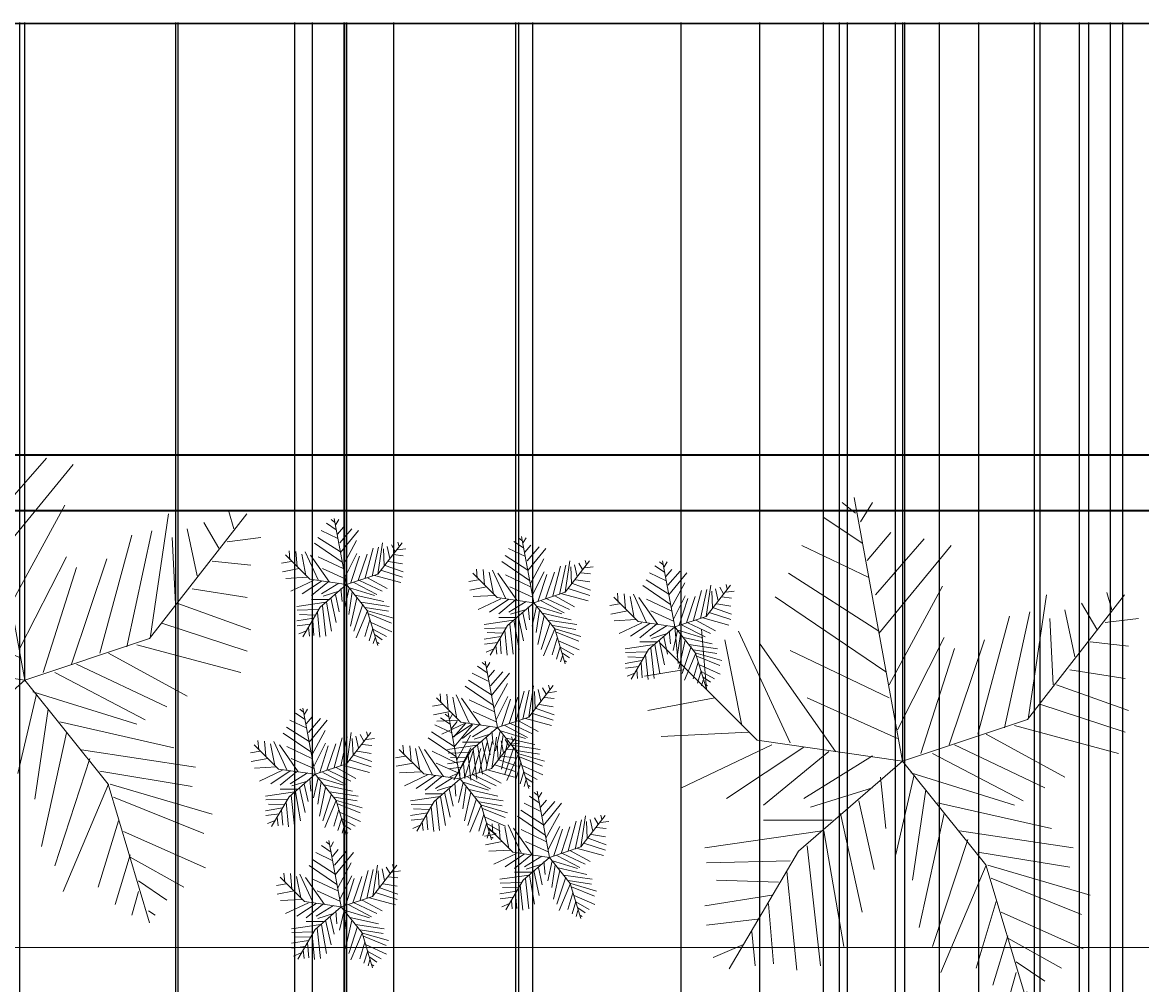
# Model space of a CAD drawing. Units: inches. Extents: x 818 to 1898, y 976 to 2364.
# Tile 81 of 96: x 1259 to 1439, y 2209 to 2364. Entities that reach past the tile are written whole.
import ezdxf

# ---------------------------------------------------------------- set-up
doc = ezdxf.new("R2010")
doc.units = ezdxf.units.IN
doc.header["$LTSCALE"] = 5
doc.header["$MEASUREMENT"] = 0
for name, color, linetype, lineweight in [('A-ANNO-DIMS', 2, 'Continuous', 18), ('C-PROP', 7, 'Continuous', 35), ('L-PLNT-BEDS', 94, 'Continuous', 18)]:
    doc.layers.add(name, color=color, linetype=linetype, lineweight=lineweight)
doc.layers.add('L-PLNT', color=116, linetype='Continuous', lineweight=13, true_color=0x136734)
doc.styles.get("Standard").update_dxf_attribs({"font": 'arial.ttf'})
doc.dimstyles.get("Standard").update_dxf_attribs({"dimtxt": 0.18, "dimasz": 0.18, "dimexe": 0.18, "dimexo": 0.0625, "dimgap": 0.09, "dimtad": 0, "dimtih": 1, "dimtoh": 1, "dimdec": 4, "dimzin": 0, "dimdsep": 46, "dimtxsty": 'Standard', "dimcen": 0.09, "dimadec": 0, "dimazin": 0, "dimtfac": 1, "dimtdec": 4, "dimtofl": 0, "dimtmove": 0, "dimatfit": 3, "dimfxl": 1, "dimtolj": 1, "dimtzin": 0, "dimarcsym": 0})

# ---------------------------------------------------------------- blocks, each defined once
blk = doc.blocks.new('SHRUB-ACCENT')
for p, q in [((8.53, 19.84), (7.99, 20.28)), ((10.44, 9.82), (8.47, 20.47)), ((8.74, 19.5), (9.21, 20.28)), ((9.08, 17.24), (6.37, 18.54)), ((8.8, 18.63), (7.25, 19.67)), ((9.01, 17.93), (9.96, 19.06)), ((9.35, 16.54), (11.31, 18.8)), ((9.48, 14.98), (12.39, 18.54)), ((9.75, 13.42), (5.28, 16.46)), ((9.48, 15.07), (5.82, 17.41)), ((9.89, 12.9), (12.06, 16.89)), ((15.49, 11.5), (19.41, 16.55)), ((15.51, 11.51), (16.25, 16.54)), ((18.69, 16.63), (18.9, 15.94)), ((4.55, 10.66), (0.62, 14.58)), ((1.35, 13.77), (1.22, 15.24)), ((2.3, 15.16), (2.51, 12.72)), ((3.25, 14.72), (3.93, 11.25)), ((3.79, 15.07), (5.89, 10.55)), ((7.72, 10.21), (4.67, 14.55)), ((10.23, 11.07), (12.12, 14.81)), ((12.33, 10.47), (13.75, 14.72)), ((13.48, 10.9), (14.76, 15.68)), ((14.56, 11.16), (15.58, 15.85)), ((16.39, 15.59), (16.53, 12.9)), ((17, 15.94), (17.41, 14.03)), ((17.68, 16.2), (18.29, 15.16)), ((18.02, 14.63), (19.57, 14.46)), ((18.62, 15.42), (19.98, 15.59)), ((1.56, 13.51), (0, 13.25)), ((5.89, 14.29), (9.89, 12.38)), ((11.17, 10.12), (12.53, 14.37)), ((16.66, 12.9), (19.57, 11.86)), ((17.2, 13.51), (19.44, 13.16)), ((2.84, 12.38), (0.14, 11.86)), ((4.2, 10.99), (0.68, 10.81)), ((6.57, 12.38), (10.23, 10.73)), ((10.44, 9.82), (15.49, 11.5)), ((13.82, 10.9), (17, 9.16)), ((14.97, 11.25), (19.17, 10.12)), ((15.98, 12.12), (19.44, 10.99)), ((5.15, 10.47), (1.49, 8.73)), ((6.43, 10.38), (3.32, 8.3)), ((10.44, 9.82), (4.55, 10.66)), ((7.45, 10.21), (4.81, 8.04)), ((10.44, 9.82), (6.23, 6.17)), ((9.21, 10.03), (6.43, 8.3)), ((9.55, 9.16), (9.75, 7.08)), ((10.9, 9.25), (10.16, 6.04)), ((10.44, 9.82), (13.8, 5.61)), ((10.77, 9.34), (14.97, 8.04)), ((11.65, 10.12), (15.31, 8.21)), ((12.53, 10.47), (16.19, 8.73)), ((7.59, 7.43), (4.81, 7.43)), ((9.21, 8.73), (6.7, 7.95)), ((7.92, 7.69), (8.8, 3.69)), ((8.67, 8.21), (9.28, 5.43)), ((11.38, 8.64), (10.84, 5)), ((12.12, 7.69), (11.11, 3.09)), ((11.85, 8.12), (16.46, 7.08)), ((7.18, 6.99), (2.44, 6.3)), ((5.89, 5.78), (2.51, 5.69)), ((6.23, 6.17), (3.43, 1.4)), ((6.57, 6.39), (7.11, 1.52)), ((7.25, 6.99), (8.06, 2.31)), ((13.07, 6.65), (11.65, 2.31)), ((13.82, 5.6), (11.99, 1.26)), ((12.73, 6.99), (17.34, 6.3)), ((13.48, 6.13), (17.2, 5.52)), ((13.8, 5.61), (15.49, 0)), ((13.88, 5.6), (18.02, 4.39)), ((5.15, 4.39), (2.44, 3.95)), ((5.42, 4.91), (2.91, 5)), ((5.01, 4.04), (5.21, 1.61)), ((5.76, 5.34), (6.16, 1.35)), ((14.22, 4.13), (13.41, 1.44)), ((14.02, 5.08), (17.68, 3.61)), ((14.43, 3.69), (17.74, 2.22)), ((4.67, 3.43), (2.51, 3.17)), ((4, 2.39), (2.78, 1.87)), ((4.33, 2.91), (4.47, 1.52)), ((14.7, 2.74), (14.09, 0.74)), ((14.7, 2.65), (16.86, 1.44)), ((15.04, 1.26), (14.76, 0.31)), ((15.04, 1.7), (16.19, 0.92)), ((15.44, 0.48), (15.71, 0.31))]:
    blk.add_line(p, q)
blk = doc.blocks.new('PALM-BORDER')
for p, q in [((41.53, 39.05), (33.72, 81.45)), ((33.95, 78.95), (31.8, 80.68)), ((34.76, 77.57), (36.65, 80.68)), ((35.03, 74.11), (28.83, 78.26)), ((35.84, 71.35), (39.61, 75.84)), ((37.18, 65.82), (45, 74.8)), ((36.11, 68.59), (25.33, 73.77)), ((37.72, 59.6), (49.31, 73.77)), ((37.72, 59.95), (23.17, 69.28)), ((39.34, 51.31), (47.96, 67.2)), ((38.8, 53.39), (21.02, 65.48)), ((61.61, 45.75), (77.23, 65.83)), ((61.71, 45.79), (64.67, 65.82)), ((74.37, 66.17), (75.18, 63.4)), ((57.93, 44.41), (61.97, 63.06)), ((67.63, 63.4), (69.25, 55.81)), ((70.33, 64.44), (72.75, 60.3)), ((53.62, 43.37), (58.74, 62.37)), ((65.21, 62.02), (65.75, 51.31)), ((74.1, 61.33), (79.49, 62.02)), ((5.39, 54.77), (4.85, 60.64)), ((9.16, 60.3), (9.97, 50.62)), ((15.09, 59.95), (23.44, 41.99)), ((18.1, 42.4), (2.48, 58.02)), ((12.93, 58.57), (15.63, 44.75)), ((30.72, 40.61), (18.59, 57.88)), ((40.69, 44.06), (48.23, 58.91)), ((49.04, 41.64), (54.7, 58.57)), ((71.68, 58.22), (77.87, 57.53)), ((23.44, 56.84), (39.34, 49.24)), ((44.46, 40.26), (49.85, 57.19)), ((6.2, 53.73), (0, 52.7)), ((68.44, 53.73), (77.33, 52.35)), ((66.29, 51.31), (77.87, 47.17)), ((11.32, 49.24), (0.54, 47.17)), ((26.14, 49.24), (40.69, 42.68)), ((63.59, 48.21), (77.33, 43.71)), ((41.53, 39.05), (61.61, 45.75)), ((16.71, 43.71), (2.69, 43.02)), ((54.97, 43.37), (67.63, 36.46)), ((59.55, 44.75), (76.26, 40.26)), ((20.48, 41.64), (5.93, 34.73)), ((41.53, 39.05), (18.1, 42.4)), ((49.85, 41.64), (64.4, 34.73)), ((25.6, 41.3), (13.2, 33.01)), ((29.64, 40.61), (19.13, 31.97)), ((36.65, 39.91), (25.6, 33.01)), ((46.35, 40.26), (60.9, 32.66)), ((41.53, 39.05), (24.79, 24.55)), ((41.53, 39.05), (54.92, 22.32)), ((37.99, 36.46), (38.8, 28.17)), ((43.38, 36.81), (40.42, 24.02)), ((42.84, 37.15), (59.55, 31.97)), ((36.65, 34.73), (26.68, 31.62)), ((45.27, 34.39), (43.11, 19.88)), ((34.49, 32.66), (36.92, 21.61)), ((47.15, 32.32), (65.48, 28.17)), ((30.18, 29.55), (19.13, 29.55)), ((31.53, 30.59), (35.03, 14.7)), ((48.23, 30.59), (44.19, 12.28)), ((28.56, 27.82), (9.7, 25.06)), ((28.83, 27.82), (32.07, 9.17)), ((50.66, 27.82), (68.98, 25.06)), ((26.14, 25.41), (28.29, 6.06)), ((52, 26.44), (46.35, 9.17)), ((24.79, 24.55), (13.63, 5.58)), ((53.62, 24.37), (68.44, 21.95)), ((23.44, 22.99), (9.97, 22.64)), ((54.97, 22.3), (47.69, 5.02)), ((54.92, 22.32), (61.61, 0)), ((55.24, 22.3), (71.68, 17.46)), ((21.56, 19.53), (11.59, 19.88)), ((22.9, 21.26), (24.52, 5.37)), ((55.78, 20.22), (70.33, 14.35)), ((20.48, 17.46), (9.7, 15.73)), ((56.59, 16.42), (53.35, 5.72)), ((19.94, 16.08), (20.75, 6.41)), ((57.39, 14.7), (70.6, 8.83)), ((18.59, 13.66), (9.97, 12.62)), ((17.24, 11.59), (17.78, 6.06)), ((58.47, 10.9), (56.05, 2.95)), ((15.9, 9.52), (11.05, 7.44)), ((58.47, 10.55), (67.09, 5.72)), ((59.82, 6.75), (64.4, 3.64)), ((59.82, 5.02), (58.74, 1.22)), ((61.44, 1.92), (62.51, 1.22))]:
    blk.add_line(p, q)
blk = doc.blocks.new('*D57')
at = {"layer": 'A-ANNO-DIMS', "color": 0, "lineweight": -2, "ltscale": 5, "transparency": 16777216}
for p, q in [((992.73, 2294.28), (992.73, 2363.87)), ((992.91, 2363.69), (1395.43, 2363.69)), ((1798.54, 2363.69), (1396.01, 2363.69)), ((1798.72, 2294.28), (1798.72, 2363.87))]:
    blk.add_line(p, q, dxfattribs=at)
at = {"layer": 'A-ANNO-DIMS', "color": 0, "ltscale": 5, "transparency": 16777216}
for points in [[(992.91, 2363.72), (992.91, 2363.66), (992.73, 2363.69)], [(1798.54, 2363.72), (1798.54, 2363.66), (1798.72, 2363.69)]]:
    blk.add_solid(points, dxfattribs=at)
at = {"layer": 'Defpoints', "color": 0, "ltscale": 5, "transparency": 16777216}
for p in [(1798.72, 2363.69), (992.73, 2294.22), (1798.72, 2294.22)]:
    blk.add_point(p, dxfattribs=at)
at = {"layer": 'A-ANNO-DIMS', "color": 0, "ltscale": 5, "transparency": 16777216, "insert": (1395.72, 2363.69), "char_height": 0.18, "attachment_point": 5}
blk.add_mtext('\\A1;806', dxfattribs=at)
blk = doc.blocks.new('*D61')
at = {"layer": 'A-ANNO-DIMS', "color": 0, "lineweight": -2, "ltscale": 5, "transparency": 16777216}
for p, q in [((1071.73, 1203.03), (1071.73, 2363.87)), ((1071.91, 2363.69), (1250.94, 2363.69)), ((1430.55, 2363.69), (1251.51, 2363.69)), ((1430.73, 1203.03), (1430.73, 2363.87))]:
    blk.add_line(p, q, dxfattribs=at)
at = {"layer": 'A-ANNO-DIMS', "color": 0, "ltscale": 5, "transparency": 16777216}
for points in [[(1071.91, 2363.72), (1071.91, 2363.66), (1071.73, 2363.69)], [(1430.55, 2363.72), (1430.55, 2363.66), (1430.73, 2363.69)]]:
    blk.add_solid(points, dxfattribs=at)
at = {"layer": 'Defpoints', "color": 0, "ltscale": 5, "transparency": 16777216}
for p in [(1430.73, 2363.69), (1071.73, 1202.96), (1430.73, 1202.96)]:
    blk.add_point(p, dxfattribs=at)
at = {"layer": 'A-ANNO-DIMS', "color": 0, "ltscale": 5, "transparency": 16777216, "insert": (1251.23, 2363.69), "char_height": 0.18, "attachment_point": 5}
blk.add_mtext('\\A1;359', dxfattribs=at)
blk = doc.blocks.new('*D64')
at = {"layer": 'A-ANNO-DIMS', "color": 0, "lineweight": -2, "ltscale": 5, "transparency": 16777216}
for p, q in [((1197.73, 1501.14), (1197.73, 2363.87)), ((1197.91, 2363.69), (1313.93, 2363.69)), ((1430.55, 2363.69), (1314.52, 2363.69)), ((1430.73, 1501.14), (1430.73, 2363.87))]:
    blk.add_line(p, q, dxfattribs=at)
at = {"layer": 'A-ANNO-DIMS', "color": 0, "ltscale": 5, "transparency": 16777216}
for points in [[(1197.91, 2363.72), (1197.91, 2363.66), (1197.73, 2363.69)], [(1430.55, 2363.72), (1430.55, 2363.66), (1430.73, 2363.69)]]:
    blk.add_solid(points, dxfattribs=at)
at = {"layer": 'Defpoints', "color": 0, "ltscale": 5, "transparency": 16777216}
for p in [(1430.73, 2363.69), (1197.73, 1501.08), (1430.73, 1501.08)]:
    blk.add_point(p, dxfattribs=at)
at = {"layer": 'A-ANNO-DIMS', "color": 0, "ltscale": 5, "transparency": 16777216, "insert": (1314.23, 2363.69), "char_height": 0.18, "attachment_point": 5}
blk.add_mtext('\\A1;233', dxfattribs=at)
blk = doc.blocks.new('*D86')
at = {"layer": 'A-ANNO-DIMS', "color": 0, "lineweight": -2, "ltscale": 5, "transparency": 16777216}
for p, q in [((1258.73, 2053.14), (1258.73, 2363.87)), ((1258.91, 2363.69), (1486.43, 2363.69)), ((1714.55, 2363.69), (1487.02, 2363.69)), ((1714.73, 2053.14), (1714.73, 2363.87))]:
    blk.add_line(p, q, dxfattribs=at)
at = {"layer": 'A-ANNO-DIMS', "color": 0, "ltscale": 5, "transparency": 16777216}
for points in [[(1258.91, 2363.72), (1258.91, 2363.66), (1258.73, 2363.69)], [(1714.55, 2363.72), (1714.55, 2363.66), (1714.73, 2363.69)]]:
    blk.add_solid(points, dxfattribs=at)
at = {"layer": 'Defpoints', "color": 0, "ltscale": 5, "transparency": 16777216}
for p in [(1714.73, 2363.69), (1258.73, 2053.08), (1714.73, 2053.08)]:
    blk.add_point(p, dxfattribs=at)
at = {"layer": 'A-ANNO-DIMS', "color": 0, "ltscale": 5, "transparency": 16777216, "insert": (1486.73, 2363.69), "char_height": 0.18, "attachment_point": 5}
blk.add_mtext('\\A1;456', dxfattribs=at)
blk = doc.blocks.new('*D96')
at = {"layer": 'A-ANNO-DIMS', "color": 0, "lineweight": -2, "ltscale": 5, "transparency": 16777216}
for p, q in [((1229.65, 1071.12), (1229.65, 2363.87)), ((1229.83, 2363.69), (1256.52, 2363.69)), ((1283.99, 2363.69), (1257.3, 2363.69)), ((1284.17, 1071.12), (1284.17, 2363.87))]:
    blk.add_line(p, q, dxfattribs=at)
at = {"layer": 'A-ANNO-DIMS', "color": 0, "ltscale": 5, "transparency": 16777216}
for points in [[(1229.83, 2363.72), (1229.83, 2363.66), (1229.65, 2363.69)], [(1283.99, 2363.72), (1283.99, 2363.66), (1284.17, 2363.69)]]:
    blk.add_solid(points, dxfattribs=at)
at = {"layer": 'Defpoints', "color": 0, "ltscale": 5, "transparency": 16777216}
for p in [(1284.17, 2363.69), (1229.65, 1071.06), (1284.17, 1071.06)]:
    blk.add_point(p, dxfattribs=at)
at = {"layer": 'A-ANNO-DIMS', "color": 0, "ltscale": 5, "transparency": 16777216, "insert": (1256.91, 2363.69), "char_height": 0.18, "attachment_point": 5}
blk.add_mtext('\\A1;54.52', dxfattribs=at)
blk = doc.blocks.new('*D97')
at = {"layer": 'A-ANNO-DIMS', "color": 0, "lineweight": -2, "ltscale": 5, "transparency": 16777216}
for p, q in [((1284.17, 1071.12), (1284.17, 2363.87)), ((1284.35, 2363.69), (1310.96, 2363.69)), ((1338.36, 2363.69), (1311.75, 2363.69)), ((1338.54, 1071.12), (1338.54, 2363.87))]:
    blk.add_line(p, q, dxfattribs=at)
at = {"layer": 'A-ANNO-DIMS', "color": 0, "ltscale": 5, "transparency": 16777216}
for points in [[(1284.35, 2363.72), (1284.35, 2363.66), (1284.17, 2363.69)], [(1338.36, 2363.72), (1338.36, 2363.66), (1338.54, 2363.69)]]:
    blk.add_solid(points, dxfattribs=at)
at = {"layer": 'Defpoints', "color": 0, "ltscale": 5, "transparency": 16777216}
for p in [(1338.54, 2363.69), (1284.17, 1071.06), (1338.54, 1071.06)]:
    blk.add_point(p, dxfattribs=at)
at = {"layer": 'A-ANNO-DIMS', "color": 0, "ltscale": 5, "transparency": 16777216, "insert": (1311.36, 2363.69), "char_height": 0.18, "attachment_point": 5}
blk.add_mtext('\\A1;54.37', dxfattribs=at)
blk = doc.blocks.new('*D98')
at = {"layer": 'A-ANNO-DIMS', "color": 0, "lineweight": -2, "ltscale": 5, "transparency": 16777216}
for p, q in [((1338.54, 1071.12), (1338.54, 2363.87)), ((1338.72, 2363.69), (1364.81, 2363.69)), ((1391.7, 2363.69), (1365.6, 2363.69)), ((1391.88, 1071.12), (1391.88, 2363.87))]:
    blk.add_line(p, q, dxfattribs=at)
at = {"layer": 'A-ANNO-DIMS', "color": 0, "ltscale": 5, "transparency": 16777216}
for points in [[(1338.72, 2363.72), (1338.72, 2363.66), (1338.54, 2363.69)], [(1391.7, 2363.72), (1391.7, 2363.66), (1391.88, 2363.69)]]:
    blk.add_solid(points, dxfattribs=at)
at = {"layer": 'Defpoints', "color": 0, "ltscale": 5, "transparency": 16777216}
for p in [(1391.88, 2363.69), (1338.54, 1071.06), (1391.88, 1071.06)]:
    blk.add_point(p, dxfattribs=at)
at = {"layer": 'A-ANNO-DIMS', "color": 0, "ltscale": 5, "transparency": 16777216, "insert": (1365.21, 2363.69), "char_height": 0.18, "attachment_point": 5}
blk.add_mtext('\\A1;53.33', dxfattribs=at)
blk = doc.blocks.new('*D99')
at = {"layer": 'A-ANNO-DIMS', "color": 0, "lineweight": -2, "ltscale": 5, "transparency": 16777216}
for p, q in [((1391.88, 1071.12), (1391.88, 2363.87)), ((1392.06, 2363.69), (1420.45, 2363.69)), ((1449.64, 2363.69), (1421.24, 2363.69)), ((1449.82, 1071.12), (1449.82, 2363.87))]:
    blk.add_line(p, q, dxfattribs=at)
at = {"layer": 'A-ANNO-DIMS', "color": 0, "ltscale": 5, "transparency": 16777216}
for points in [[(1392.06, 2363.72), (1392.06, 2363.66), (1391.88, 2363.69)], [(1449.64, 2363.72), (1449.64, 2363.66), (1449.82, 2363.69)]]:
    blk.add_solid(points, dxfattribs=at)
at = {"layer": 'Defpoints', "color": 0, "ltscale": 5, "transparency": 16777216}
for p in [(1449.82, 2363.69), (1391.88, 1071.06), (1449.82, 1071.06)]:
    blk.add_point(p, dxfattribs=at)
at = {"layer": 'A-ANNO-DIMS', "color": 0, "ltscale": 5, "transparency": 16777216, "insert": (1420.85, 2363.69), "char_height": 0.18, "attachment_point": 5}
blk.add_mtext('\\A1;57.94', dxfattribs=at)
blk = doc.blocks.new('*D136')
at = {"layer": 'A-ANNO-DIMS', "color": 0, "lineweight": -2, "ltscale": 5, "transparency": 16777216}
for p, q in [((1151.43, 2252.7), (1151.43, 2363.87)), ((1151.61, 2363.69), (1205.1, 2363.69)), ((1259.34, 2363.69), (1205.84, 2363.69)), ((1259.52, 2258.06), (1259.52, 2363.87))]:
    blk.add_line(p, q, dxfattribs=at)
at = {"layer": 'A-ANNO-DIMS', "color": 0, "ltscale": 5, "transparency": 16777216}
for points in [[(1151.61, 2363.72), (1151.61, 2363.66), (1151.43, 2363.69)], [(1259.34, 2363.72), (1259.34, 2363.66), (1259.52, 2363.69)]]:
    blk.add_solid(points, dxfattribs=at)
at = {"layer": 'Defpoints', "color": 0, "ltscale": 5, "transparency": 16777216}
for p in [(1259.52, 2363.69), (1259.52, 2257.99), (1151.43, 2252.64)]:
    blk.add_point(p, dxfattribs=at)
at = {"layer": 'A-ANNO-DIMS', "color": 0, "ltscale": 5, "transparency": 16777216, "insert": (1205.47, 2363.69), "char_height": 0.18, "attachment_point": 5}
blk.add_mtext('\\A1;108.1', dxfattribs=at)
blk = doc.blocks.new('*D137')
at = {"layer": 'A-ANNO-DIMS', "color": 0, "lineweight": -2, "ltscale": 5, "transparency": 16777216}
for p, q in [((1259.52, 2258.06), (1259.52, 2363.87)), ((1259.7, 2363.69), (1329.69, 2363.69)), ((1400.6, 2363.69), (1330.6, 2363.69)), ((1400.78, 2245.03), (1400.78, 2363.87))]:
    blk.add_line(p, q, dxfattribs=at)
at = {"layer": 'A-ANNO-DIMS', "color": 0, "ltscale": 5, "transparency": 16777216}
for points in [[(1259.7, 2363.72), (1259.7, 2363.66), (1259.52, 2363.69)], [(1400.6, 2363.72), (1400.6, 2363.66), (1400.78, 2363.69)]]:
    blk.add_solid(points, dxfattribs=at)
at = {"layer": 'Defpoints', "color": 0, "ltscale": 5, "transparency": 16777216}
for p in [(1400.78, 2363.69), (1259.52, 2257.99), (1400.78, 2244.97)]:
    blk.add_point(p, dxfattribs=at)
at = {"layer": 'A-ANNO-DIMS', "color": 0, "ltscale": 5, "transparency": 16777216, "insert": (1330.15, 2363.69), "char_height": 0.18, "attachment_point": 5}
blk.add_mtext('\\A1;141.26', dxfattribs=at)
blk = doc.blocks.new('*D138')
at = {"layer": 'A-ANNO-DIMS', "color": 0, "lineweight": -2, "ltscale": 5, "transparency": 16777216}
for p, q in [((1400.78, 2245.03), (1400.78, 2363.87)), ((1400.96, 2363.69), (1475.45, 2363.69)), ((1550.69, 2363.69), (1476.19, 2363.69)), ((1550.87, 2253.22), (1550.87, 2363.87))]:
    blk.add_line(p, q, dxfattribs=at)
at = {"layer": 'A-ANNO-DIMS', "color": 0, "ltscale": 5, "transparency": 16777216}
for points in [[(1400.96, 2363.72), (1400.96, 2363.66), (1400.78, 2363.69)], [(1550.69, 2363.72), (1550.69, 2363.66), (1550.87, 2363.69)]]:
    blk.add_solid(points, dxfattribs=at)
at = {"layer": 'Defpoints', "color": 0, "ltscale": 5, "transparency": 16777216}
for p in [(1550.87, 2363.69), (1550.87, 2253.16), (1400.78, 2244.97)]:
    blk.add_point(p, dxfattribs=at)
at = {"layer": 'A-ANNO-DIMS', "color": 0, "ltscale": 5, "transparency": 16777216, "insert": (1475.82, 2363.69), "char_height": 0.18, "attachment_point": 5}
blk.add_mtext('\\A1;150.1', dxfattribs=at)
blk = doc.blocks.new('*D161')
at = {"layer": 'A-ANNO-DIMS', "color": 0, "lineweight": -2, "ltscale": 5, "transparency": 16777216}
for p, q in [((1429.23, 1876.14), (1429.23, 2363.87)), ((1429.41, 2363.69), (1509.59, 2363.69)), ((1590.55, 2363.69), (1510.36, 2363.69)), ((1590.73, 1876.14), (1590.73, 2363.87))]:
    blk.add_line(p, q, dxfattribs=at)
at = {"layer": 'A-ANNO-DIMS', "color": 0, "ltscale": 5, "transparency": 16777216}
for points in [[(1429.41, 2363.72), (1429.41, 2363.66), (1429.23, 2363.69)], [(1590.55, 2363.72), (1590.55, 2363.66), (1590.73, 2363.69)]]:
    blk.add_solid(points, dxfattribs=at)
at = {"layer": 'Defpoints', "color": 0, "ltscale": 5, "transparency": 16777216}
for p in [(1590.73, 2363.69), (1429.23, 1876.08), (1590.73, 1876.08)]:
    blk.add_point(p, dxfattribs=at)
at = {"layer": 'A-ANNO-DIMS', "color": 0, "ltscale": 5, "transparency": 16777216, "insert": (1509.98, 2363.69), "char_height": 0.18, "attachment_point": 5}
blk.add_mtext('\\A1;161.5', dxfattribs=at)
blk = doc.blocks.new('*D165')
at = {"layer": 'A-ANNO-DIMS', "color": 0, "lineweight": -2, "ltscale": 5, "transparency": 16777216}
for p, q in [((1283.82, 1510.14), (1283.82, 2363.87)), ((1284, 2363.69), (1324.09, 2363.69)), ((1364.97, 2363.69), (1324.88, 2363.69)), ((1365.15, 1510.14), (1365.15, 2363.87))]:
    blk.add_line(p, q, dxfattribs=at)
at = {"layer": 'A-ANNO-DIMS', "color": 0, "ltscale": 5, "transparency": 16777216}
for points in [[(1284, 2363.72), (1284, 2363.66), (1283.82, 2363.69)], [(1364.97, 2363.72), (1364.97, 2363.66), (1365.15, 2363.69)]]:
    blk.add_solid(points, dxfattribs=at)
at = {"layer": 'Defpoints', "color": 0, "ltscale": 5, "transparency": 16777216}
for p in [(1365.15, 2363.69), (1283.82, 1510.08), (1365.15, 1510.08)]:
    blk.add_point(p, dxfattribs=at)
at = {"layer": 'A-ANNO-DIMS', "color": 0, "ltscale": 5, "transparency": 16777216, "insert": (1324.48, 2363.69), "char_height": 0.18, "attachment_point": 5}
blk.add_mtext('\\A1;81.33', dxfattribs=at)
blk = doc.blocks.new('*D166')
at = {"layer": 'A-ANNO-DIMS', "color": 0, "lineweight": -2, "ltscale": 5, "transparency": 16777216}
for p, q in [((1401.15, 1510.14), (1401.15, 2363.87)), ((1401.33, 2363.69), (1415.54, 2363.69)), ((1430.55, 2363.69), (1416.33, 2363.69)), ((1430.73, 1510.14), (1430.73, 2363.87))]:
    blk.add_line(p, q, dxfattribs=at)
at = {"layer": 'A-ANNO-DIMS', "color": 0, "ltscale": 5, "transparency": 16777216}
for points in [[(1401.33, 2363.72), (1401.33, 2363.66), (1401.15, 2363.69)], [(1430.55, 2363.72), (1430.55, 2363.66), (1430.73, 2363.69)]]:
    blk.add_solid(points, dxfattribs=at)
at = {"layer": 'Defpoints', "color": 0, "ltscale": 5, "transparency": 16777216}
for p in [(1430.73, 2363.69), (1401.15, 1510.08), (1430.73, 1510.08)]:
    blk.add_point(p, dxfattribs=at)
at = {"layer": 'A-ANNO-DIMS', "color": 0, "ltscale": 5, "transparency": 16777216, "insert": (1415.94, 2363.69), "char_height": 0.18, "attachment_point": 5}
blk.add_mtext('\\A1;29.58', dxfattribs=at)
blk = doc.blocks.new('*D191')
at = {"layer": 'A-ANNO-DIMS', "color": 0, "lineweight": -2, "ltscale": 5, "transparency": 16777216}
for p, q in [((1434.23, 1409.11), (1434.23, 2363.87)), ((1434.41, 2363.69), (1435.08, 2363.69)), ((1436.05, 2363.69), (1435.37, 2363.69)), ((1436.23, 1409.11), (1436.23, 2363.87))]:
    blk.add_line(p, q, dxfattribs=at)
at = {"layer": 'A-ANNO-DIMS', "color": 0, "ltscale": 5, "transparency": 16777216}
for points in [[(1434.41, 2363.72), (1434.41, 2363.66), (1434.23, 2363.69)], [(1436.05, 2363.72), (1436.05, 2363.66), (1436.23, 2363.69)]]:
    blk.add_solid(points, dxfattribs=at)
at = {"layer": 'Defpoints', "color": 0, "ltscale": 5, "transparency": 16777216}
for p in [(1436.23, 2363.69), (1434.23, 1409.05), (1436.23, 1409.05)]:
    blk.add_point(p, dxfattribs=at)
at = {"layer": 'A-ANNO-DIMS', "color": 0, "ltscale": 5, "transparency": 16777216, "insert": (1435.23, 2363.69), "char_height": 0.18, "attachment_point": 5}
blk.add_mtext('\\A1;2', dxfattribs=at)
blk = doc.blocks.new('*D235')
at = {"layer": 'A-ANNO-DIMS', "color": 0, "lineweight": -2, "ltscale": 5, "transparency": 16777216}
for p, q in [((1310.91, 2026.27), (1310.91, 2363.87)), ((1311.09, 2363.69), (1324.48, 2363.69)), ((1338.81, 2363.69), (1325.41, 2363.69)), ((1338.99, 2026.27), (1338.99, 2363.87))]:
    blk.add_line(p, q, dxfattribs=at)
at = {"layer": 'A-ANNO-DIMS', "color": 0, "ltscale": 5, "transparency": 16777216}
for points in [[(1311.09, 2363.72), (1311.09, 2363.66), (1310.91, 2363.69)], [(1338.81, 2363.72), (1338.81, 2363.66), (1338.99, 2363.69)]]:
    blk.add_solid(points, dxfattribs=at)
at = {"layer": 'Defpoints', "color": 0, "ltscale": 5, "transparency": 16777216}
for p in [(1338.99, 2363.69), (1310.91, 2026.21), (1338.99, 2026.21)]:
    blk.add_point(p, dxfattribs=at)
at = {"layer": 'A-ANNO-DIMS', "color": 0, "ltscale": 5, "transparency": 16777216, "insert": (1324.95, 2363.69), "char_height": 0.18, "attachment_point": 5}
blk.add_mtext('\\A1;28.084', dxfattribs=at)
blk = doc.blocks.new('*D255')
at = {"layer": 'A-ANNO-DIMS', "color": 0, "lineweight": -2, "ltscale": 5, "transparency": 16777216}
for p, q in [((1388.03, 2053.14), (1388.03, 2363.87)), ((1388.21, 2363.69), (1388.94, 2363.69)), ((1390.46, 2363.69), (1389.73, 2363.69)), ((1390.64, 2053.14), (1390.64, 2363.87))]:
    blk.add_line(p, q, dxfattribs=at)
at = {"layer": 'A-ANNO-DIMS', "color": 0, "ltscale": 5, "transparency": 16777216}
for points in [[(1388.21, 2363.72), (1388.21, 2363.66), (1388.03, 2363.69)], [(1390.46, 2363.72), (1390.46, 2363.66), (1390.64, 2363.69)]]:
    blk.add_solid(points, dxfattribs=at)
at = {"layer": 'Defpoints', "color": 0, "ltscale": 5, "transparency": 16777216}
for p in [(1390.64, 2363.69), (1388.03, 2053.08), (1390.64, 2053.08)]:
    blk.add_point(p, dxfattribs=at)
at = {"layer": 'A-ANNO-DIMS', "color": 0, "ltscale": 5, "transparency": 16777216, "insert": (1389.33, 2363.69), "char_height": 0.18, "attachment_point": 5}
blk.add_mtext('\\A1;2.604', dxfattribs=at)
blk = doc.blocks.new('*D256')
at = {"layer": 'A-ANNO-DIMS', "color": 0, "lineweight": -2, "ltscale": 5, "transparency": 16777216}
for p, q in [((1399.64, 2053.14), (1399.64, 2363.87)), ((1399.82, 2363.69), (1405.87, 2363.69)), ((1412.84, 2363.69), (1406.78, 2363.69)), ((1413.02, 2077.25), (1413.02, 2363.87))]:
    blk.add_line(p, q, dxfattribs=at)
at = {"layer": 'A-ANNO-DIMS', "color": 0, "ltscale": 5, "transparency": 16777216}
for points in [[(1399.82, 2363.72), (1399.82, 2363.66), (1399.64, 2363.69)], [(1412.84, 2363.72), (1412.84, 2363.66), (1413.02, 2363.69)]]:
    blk.add_solid(points, dxfattribs=at)
at = {"layer": 'Defpoints', "color": 0, "ltscale": 5, "transparency": 16777216}
for p in [(1413.02, 2363.69), (1413.02, 2077.19), (1399.64, 2053.08)]:
    blk.add_point(p, dxfattribs=at)
at = {"layer": 'A-ANNO-DIMS', "color": 0, "ltscale": 5, "transparency": 16777216, "insert": (1406.33, 2363.69), "char_height": 0.18, "attachment_point": 5}
blk.add_mtext('\\A1;13.384', dxfattribs=at)
blk = doc.blocks.new('*D258')
at = {"layer": 'A-ANNO-DIMS', "color": 0, "lineweight": -2, "ltscale": 5, "transparency": 16777216}
for p, q in [((1422.02, 2053.14), (1422.02, 2363.87)), ((1422.2, 2363.69), (1453.26, 2363.69)), ((1484.94, 2363.69), (1453.88, 2363.69)), ((1485.12, 2053.14), (1485.12, 2363.87))]:
    blk.add_line(p, q, dxfattribs=at)
at = {"layer": 'A-ANNO-DIMS', "color": 0, "ltscale": 5, "transparency": 16777216}
for points in [[(1422.2, 2363.72), (1422.2, 2363.66), (1422.02, 2363.69)], [(1484.94, 2363.72), (1484.94, 2363.66), (1485.12, 2363.69)]]:
    blk.add_solid(points, dxfattribs=at)
at = {"layer": 'Defpoints', "color": 0, "ltscale": 5, "transparency": 16777216}
for p in [(1485.12, 2363.69), (1422.02, 2053.08), (1485.12, 2053.08)]:
    blk.add_point(p, dxfattribs=at)
at = {"layer": 'A-ANNO-DIMS', "color": 0, "ltscale": 5, "transparency": 16777216, "insert": (1453.57, 2363.69), "char_height": 0.18, "attachment_point": 5}
blk.add_mtext('\\A1;63.1', dxfattribs=at)
blk = doc.blocks.new('*D269')
at = {"layer": 'A-ANNO-DIMS', "color": 0, "lineweight": -2, "ltscale": 5, "transparency": 16777216}
for p, q in [((1246.94, 1534.14), (1246.94, 2363.87)), ((1247.12, 2363.69), (1293.71, 2363.69)), ((1341.08, 2363.69), (1294.49, 2363.69)), ((1341.26, 1534.14), (1341.26, 2363.87))]:
    blk.add_line(p, q, dxfattribs=at)
at = {"layer": 'A-ANNO-DIMS', "color": 0, "ltscale": 5, "transparency": 16777216}
for points in [[(1247.12, 2363.72), (1247.12, 2363.66), (1246.94, 2363.69)], [(1341.08, 2363.72), (1341.08, 2363.66), (1341.26, 2363.69)]]:
    blk.add_solid(points, dxfattribs=at)
at = {"layer": 'Defpoints', "color": 0, "ltscale": 5, "transparency": 16777216}
for p in [(1341.26, 2363.69), (1246.94, 1534.08), (1341.26, 1534.08)]:
    blk.add_point(p, dxfattribs=at)
at = {"layer": 'A-ANNO-DIMS', "color": 0, "ltscale": 5, "transparency": 16777216, "insert": (1294.1, 2363.69), "char_height": 0.18, "attachment_point": 5}
blk.add_mtext('\\A1;94.32', dxfattribs=at)
blk = doc.blocks.new('*D273')
at = {"layer": 'A-ANNO-DIMS', "color": 0, "lineweight": -2, "ltscale": 5, "transparency": 16777216}
for p, q in [((1406.73, 1587.48), (1406.73, 2363.87)), ((1406.91, 2363.69), (1418.51, 2363.69)), ((1430.55, 2363.69), (1418.95, 2363.69)), ((1430.73, 1587.48), (1430.73, 2363.87))]:
    blk.add_line(p, q, dxfattribs=at)
at = {"layer": 'A-ANNO-DIMS', "color": 0, "ltscale": 5, "transparency": 16777216}
for points in [[(1406.91, 2363.72), (1406.91, 2363.66), (1406.73, 2363.69)], [(1430.55, 2363.72), (1430.55, 2363.66), (1430.73, 2363.69)]]:
    blk.add_solid(points, dxfattribs=at)
at = {"layer": 'Defpoints', "color": 0, "ltscale": 5, "transparency": 16777216}
for p in [(1430.73, 2363.69), (1406.73, 1587.42), (1430.73, 1587.42)]:
    blk.add_point(p, dxfattribs=at)
at = {"layer": 'A-ANNO-DIMS', "color": 0, "ltscale": 5, "transparency": 16777216, "insert": (1418.73, 2363.69), "char_height": 0.18, "attachment_point": 5}
blk.add_mtext('\\A1;24', dxfattribs=at)
blk = doc.blocks.new('*D274')
at = {"layer": 'A-ANNO-DIMS', "color": 0, "lineweight": -2, "ltscale": 5, "transparency": 16777216}
for p, q in [((1311.03, 1897.93), (1311.03, 2363.87)), ((1311.21, 2363.69), (1344.01, 2363.69)), ((1377.6, 2363.69), (1344.8, 2363.69)), ((1377.78, 1897.93), (1377.78, 2363.87))]:
    blk.add_line(p, q, dxfattribs=at)
at = {"layer": 'A-ANNO-DIMS', "color": 0, "ltscale": 5, "transparency": 16777216}
for points in [[(1311.21, 2363.72), (1311.21, 2363.66), (1311.03, 2363.69)], [(1377.6, 2363.72), (1377.6, 2363.66), (1377.78, 2363.69)]]:
    blk.add_solid(points, dxfattribs=at)
at = {"layer": 'Defpoints', "color": 0, "ltscale": 5, "transparency": 16777216}
for p in [(1377.78, 2363.69), (1311.03, 1897.87), (1377.78, 1897.87)]:
    blk.add_point(p, dxfattribs=at)
at = {"layer": 'A-ANNO-DIMS', "color": 0, "ltscale": 5, "transparency": 16777216, "insert": (1344.4, 2363.69), "char_height": 0.18, "attachment_point": 5}
blk.add_mtext('\\A1;66.75', dxfattribs=at)
blk = doc.blocks.new('*D281')
at = {"layer": 'A-ANNO-DIMS', "color": 0, "lineweight": -2, "ltscale": 5, "transparency": 16777216}
for p, q in [((1250.3, 1913.7), (1250.3, 2363.87)), ((1250.48, 2363.69), (1420.12, 2363.69)), ((1590.55, 2363.69), (1420.91, 2363.69)), ((1590.73, 2011.14), (1590.73, 2363.87))]:
    blk.add_line(p, q, dxfattribs=at)
at = {"layer": 'A-ANNO-DIMS', "color": 0, "ltscale": 5, "transparency": 16777216}
for points in [[(1250.48, 2363.72), (1250.48, 2363.66), (1250.3, 2363.69)], [(1590.55, 2363.72), (1590.55, 2363.66), (1590.73, 2363.69)]]:
    blk.add_solid(points, dxfattribs=at)
at = {"layer": 'Defpoints', "color": 0, "ltscale": 5, "transparency": 16777216}
for p in [(1590.73, 2363.69), (1590.73, 2011.08), (1250.3, 1913.64)]:
    blk.add_point(p, dxfattribs=at)
at = {"layer": 'A-ANNO-DIMS', "color": 0, "ltscale": 5, "transparency": 16777216, "insert": (1420.51, 2363.69), "char_height": 0.18, "attachment_point": 5}
blk.add_mtext('\\A1;340.4', dxfattribs=at)
blk = doc.blocks.new('*D286')
at = {"layer": 'A-ANNO-DIMS', "color": 0, "lineweight": -2, "ltscale": 5, "transparency": 16777216}
for p, q in [((1305.83, 1851.97), (1305.83, 2363.87)), ((1306.01, 2363.69), (1308.18, 2363.69)), ((1311.15, 2363.69), (1308.97, 2363.69)), ((1311.33, 1853.81), (1311.33, 2363.87))]:
    blk.add_line(p, q, dxfattribs=at)
at = {"layer": 'A-ANNO-DIMS', "color": 0, "ltscale": 5, "transparency": 16777216}
for points in [[(1306.01, 2363.72), (1306.01, 2363.66), (1305.83, 2363.69)], [(1311.15, 2363.72), (1311.15, 2363.66), (1311.33, 2363.69)]]:
    blk.add_solid(points, dxfattribs=at)
at = {"layer": 'Defpoints', "color": 0, "ltscale": 5, "transparency": 16777216}
for p in [(1305.83, 2363.69), (1311.33, 1853.75), (1305.83, 1851.91)]:
    blk.add_point(p, dxfattribs=at)
at = {"layer": 'A-ANNO-DIMS', "color": 0, "ltscale": 5, "transparency": 16777216, "insert": (1308.58, 2363.69), "char_height": 0.18, "attachment_point": 5}
blk.add_mtext('\\A1;5.499', dxfattribs=at)
blk = doc.blocks.new('*D288')
at = {"layer": 'A-ANNO-DIMS', "color": 0, "lineweight": -2, "ltscale": 5, "transparency": 16777216}
for p, q in [((1422.88, 1742.67), (1422.88, 2363.87)), ((1423.06, 2363.69), (1466.91, 2363.69)), ((1511.55, 2363.69), (1467.69, 2363.69)), ((1511.73, 1716.11), (1511.73, 2363.87))]:
    blk.add_line(p, q, dxfattribs=at)
at = {"layer": 'A-ANNO-DIMS', "color": 0, "ltscale": 5, "transparency": 16777216}
for points in [[(1423.06, 2363.72), (1423.06, 2363.66), (1422.88, 2363.69)], [(1511.55, 2363.72), (1511.55, 2363.66), (1511.73, 2363.69)]]:
    blk.add_solid(points, dxfattribs=at)
at = {"layer": 'Defpoints', "color": 0, "ltscale": 5, "transparency": 16777216}
for p in [(1511.73, 2363.69), (1422.88, 1742.61), (1511.73, 1716.05)]:
    blk.add_point(p, dxfattribs=at)
at = {"layer": 'A-ANNO-DIMS', "color": 0, "ltscale": 5, "transparency": 16777216, "insert": (1467.3, 2363.69), "char_height": 0.18, "attachment_point": 5}
blk.add_mtext('\\A1;88.85', dxfattribs=at)
blk = doc.blocks.new('*D290')
at = {"layer": 'A-ANNO-DIMS', "color": 0, "lineweight": -2, "ltscale": 5, "transparency": 16777216}
for p, q in [((1302.98, 1599.43), (1302.98, 2363.87)), ((1303.16, 2363.69), (1310.57, 2363.69)), ((1318.71, 2363.69), (1311.31, 2363.69)), ((1318.89, 1607.83), (1318.89, 2363.87))]:
    blk.add_line(p, q, dxfattribs=at)
at = {"layer": 'A-ANNO-DIMS', "color": 0, "ltscale": 5, "transparency": 16777216}
for points in [[(1303.16, 2363.72), (1303.16, 2363.66), (1302.98, 2363.69)], [(1318.71, 2363.72), (1318.71, 2363.66), (1318.89, 2363.69)]]:
    blk.add_solid(points, dxfattribs=at)
at = {"layer": 'Defpoints', "color": 0, "ltscale": 5, "transparency": 16777216}
for p in [(1318.89, 2363.69), (1318.89, 1607.77), (1302.98, 1599.37)]:
    blk.add_point(p, dxfattribs=at)
at = {"layer": 'A-ANNO-DIMS', "color": 0, "ltscale": 5, "transparency": 16777216, "insert": (1310.94, 2363.69), "char_height": 0.18, "attachment_point": 5}
blk.add_mtext('\\A1;15.91', dxfattribs=at)

msp = doc.modelspace()

# ---------------------------------------------------------------- linework, layer by layer
at = {"layer": 'C-PROP', "ltscale": 5}
for p, q in [((1798.7173, 2294.2171), (992.7251, 2294.2171)), ((1789.7173, 2285.2171), (1001.7252, 2285.2171))]:
    msp.add_line(p, q, dxfattribs=at)
at = {"layer": 'L-PLNT-BEDS', "ltscale": 5}
msp.add_line((1789.7173, 2214.9709), (1071.7251, 2214.9709), dxfattribs=at)

# ---------------------------------------------------------------- block references
at = {"layer": 'L-PLNT'}
for name, p in [('PALM-BORDER', (1217.9881, 2218.9437)), ('PALM-BORDER', (1359.2483, 2205.9177)), ('SHRUB-ACCENT', (1300.8289, 2263.5633)), ('SHRUB-ACCENT', (1330.9788, 2260.6345)), ('SHRUB-ACCENT', (1353.661, 2256.7436)), ('SHRUB-ACCENT', (1325.1163, 2240.551)), ('SHRUB-ACCENT', (1295.8039, 2233.0197)), ('SHRUB-ACCENT', (1319.1485, 2232.259)), ('SHRUB-ACCENT', (1333.4913, 2219.6306)), ('SHRUB-ACCENT', (1299.9914, 2211.6809))]:
    msp.add_blockref(name, p, dxfattribs=at)

# ---------------------------------------------------------------- dimensions: what is measured, and where the dimension line sits
at = {"layer": 'A-ANNO-DIMS', "ltscale": 5}
for base, p1, p2, override, picture, middle in [((1798.7173, 2363.6929), (992.7251, 2294.2171), (1798.7173, 2294.2171), {"dimdec": 0, "dimlfac": 1, "dimrnd": 0, "dimzin": 0, "dimdsep": 46, "dimlunit": 2}, '*D57', (1395.7212, 2363.6929)), ((1430.7251, 2363.6929), (1071.7251, 1202.9642), (1430.7251, 1202.9642), {"dimdec": 0, "dimlfac": 1, "dimrnd": 0, "dimzin": 0, "dimdsep": 46, "dimlunit": 2}, '*D61', (1251.2251, 2363.6929)), ((1259.5159, 2363.6929), (1151.4251, 2252.6408), (1259.5159, 2257.9948), {"dimdec": 1, "dimlfac": 1, "dimrnd": 0, "dimzin": 0, "dimdsep": 46, "dimlunit": 2}, '*D136', (1205.4705, 2363.6929)), ((1430.7251, 2363.6929), (1197.7251, 1501.0782), (1430.7251, 1501.0782), {"dimdec": 0, "dimlfac": 1, "dimrnd": 0, "dimzin": 0, "dimdsep": 46, "dimlunit": 2}, '*D64', (1314.2251, 2363.6929)), ((1284.1697, 2363.6929), (1229.6474, 1071.0552), (1284.1697, 1071.0552), {"dimdec": 2, "dimlfac": 1, "dimrnd": 0, "dimzin": 0, "dimdsep": 46, "dimlunit": 2}, '*D96', (1256.9085, 2363.6929)), ((1341.2593, 2363.6929), (1246.9377, 1534.0782), (1341.2593, 1534.0782), {"dimdec": 2, "dimlfac": 1, "dimrnd": 0, "dimzin": 0, "dimdsep": 46, "dimlunit": 2}, '*D269', (1294.0985, 2363.6929)), ((1590.7251, 2363.6929), (1250.3029, 1913.6401), (1590.7251, 2011.0782), {"dimdec": 1, "dimlfac": 1, "dimrnd": 0, "dimzin": 0, "dimdsep": 46, "dimlunit": 2}, '*D281', (1420.514, 2363.6929)), ((1714.7251, 2363.6929), (1258.7251, 2053.0782), (1714.7251, 2053.0782), {"dimdec": 0, "dimlfac": 1, "dimrnd": 0, "dimzin": 0, "dimdsep": 46, "dimlunit": 2}, '*D86', (1486.7251, 2363.6929)), ((1400.7761, 2363.6929), (1259.5159, 2257.9948), (1400.7761, 2244.9688), {"dimdec": 2, "dimlfac": 1, "dimrnd": 0, "dimzin": 0, "dimdsep": 46, "dimlunit": 2}, '*D137', (1330.146, 2363.6929)), ((1365.1463, 2363.6929), (1283.8183, 1510.0782), (1365.1463, 1510.0782), {"dimdec": 2, "dimlfac": 1, "dimrnd": 0, "dimzin": 0, "dimdsep": 46, "dimlunit": 2}, '*D165', (1324.4823, 2363.6929)), ((1338.5412, 2363.6929), (1284.1697, 1071.0552), (1338.5412, 1071.0552), {"dimdec": 2, "dimlfac": 1, "dimrnd": 0, "dimzin": 0, "dimdsep": 46, "dimlunit": 2}, '*D97', (1311.3554, 2363.6929)), ((1318.8931, 2363.6929), (1302.9835, 1599.3725), (1318.8931, 1607.7707), {"dimdec": 2, "dimlfac": 1, "dimrnd": 0, "dimzin": 0, "dimdsep": 46, "dimlunit": 2}, '*D290', (1310.9383, 2363.6929)), ((1305.8278, 2363.6929), (1311.3271, 1853.7496), (1305.8278, 1851.9081), {"dimdec": 3, "dimlfac": 1, "dimrnd": 0, "dimzin": 0, "dimdsep": 46, "dimlunit": 2}, '*D286', (1308.5774, 2363.6929)), ((1338.9915, 2363.6929), (1310.9077, 2026.2074), (1338.9915, 2026.2074), {"dimdec": 3, "dimlfac": 1, "dimrnd": 0, "dimzin": 0, "dimdsep": 46, "dimlunit": 2}, '*D235', (1324.9496, 2363.6929)), ((1377.7791, 2363.6929), (1311.025, 1897.8663), (1377.7791, 1897.8663), {"dimdec": 2, "dimlfac": 1, "dimrnd": 0, "dimzin": 0, "dimdsep": 46, "dimlunit": 2}, '*D274', (1344.4021, 2363.6929)), ((1391.8757, 2363.6929), (1338.5412, 1071.0552), (1391.8757, 1071.0552), {"dimdec": 2, "dimlfac": 1, "dimrnd": 0, "dimzin": 0, "dimdsep": 46, "dimlunit": 2}, '*D98', (1365.2084, 2363.6929)), ((1390.6356, 2363.6929), (1388.0315, 2053.0782), (1390.6356, 2053.0782), {"dimdec": 3, "dimlfac": 1, "dimrnd": 0, "dimzin": 0, "dimdsep": 46, "dimlunit": 2}, '*D255', (1389.3335, 2363.6929)), ((1449.8196, 2363.6929), (1391.8757, 1071.0552), (1449.8196, 1071.0552), {"dimdec": 2, "dimlfac": 1, "dimrnd": 0, "dimzin": 0, "dimdsep": 46, "dimlunit": 2}, '*D99', (1420.8477, 2363.6929)), ((1413.02, 2363.6929), (1399.6356, 2053.0782), (1413.02, 2077.1881), {"dimdec": 3, "dimlfac": 1, "dimrnd": 0, "dimzin": 0, "dimdsep": 46, "dimlunit": 2}, '*D256', (1406.3278, 2363.6929)), ((1550.8651, 2363.6929), (1400.7761, 2244.9688), (1550.8651, 2253.1602), {"dimdec": 1, "dimlfac": 1, "dimrnd": 0, "dimzin": 0, "dimdsep": 46, "dimlunit": 2}, '*D138', (1475.8206, 2363.6929)), ((1430.7251, 2363.6929), (1401.1463, 1510.0782), (1430.7251, 1510.0782), {"dimdec": 2, "dimlfac": 1, "dimrnd": 0, "dimzin": 0, "dimdsep": 46, "dimlunit": 2}, '*D166', (1415.9357, 2363.6929)), ((1430.7251, 2363.6929), (1406.7251, 1587.4164), (1430.7251, 1587.4164), {"dimdec": 0, "dimlfac": 1, "dimrnd": 0, "dimzin": 0, "dimdsep": 46, "dimlunit": 2}, '*D273', (1418.7251, 2363.6929)), ((1485.1216, 2363.6929), (1422.02, 2053.0782), (1485.1216, 2053.0782), {"dimdec": 1, "dimlfac": 1, "dimrnd": 0, "dimzin": 0, "dimdsep": 46, "dimlunit": 2}, '*D258', (1453.5708, 2363.6929)), ((1511.7251, 2363.6929), (1422.8756, 1742.6113), (1511.7251, 1716.0454), {"dimdec": 2, "dimlfac": 1, "dimrnd": 0, "dimzin": 0, "dimdsep": 46, "dimlunit": 2}, '*D288', (1467.3004, 2363.6929)), ((1590.7251, 2363.6929), (1429.2251, 1876.0782), (1590.7251, 1876.0782), {"dimdec": 1, "dimlfac": 1, "dimrnd": 0, "dimzin": 0, "dimdsep": 46, "dimlunit": 2}, '*D161', (1509.9751, 2363.6929)), ((1436.2251, 2363.6929), (1434.2251, 1409.0522), (1436.2251, 1409.0522), {"dimdec": 0, "dimlfac": 1, "dimrnd": 0, "dimzin": 0, "dimdsep": 46, "dimlunit": 2}, '*D191', (1435.2251, 2363.6929))]:
    dim = msp.add_linear_dim(base=base, p1=p1, p2=p2, dimstyle='Standard', override=override, dxfattribs=at)
    dim.commit()
    dim.dimension.update_dxf_attribs({"geometry": picture, "text_midpoint": middle})

doc.saveas('drawing.dxf')
